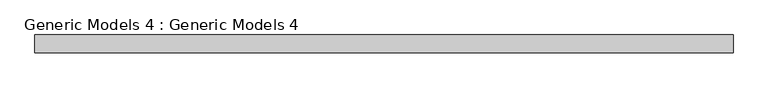
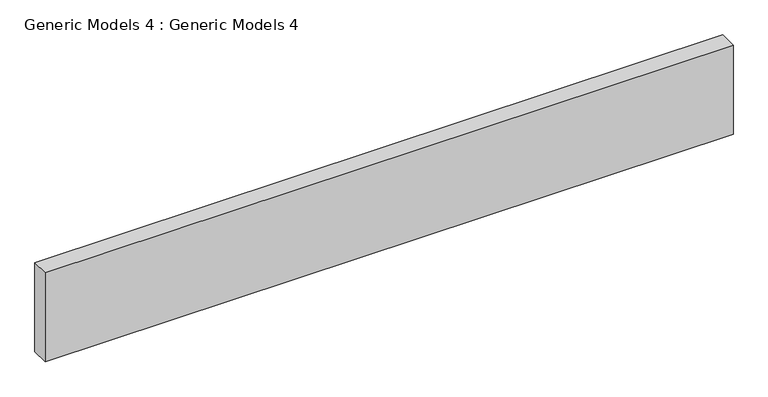
"""IFC4 building model written with IfcOpenShell, lengths in millimetres: proxy geometry, Generic Models 4 : Generic Models 4."""

from ifc_helpers import new_model, si_unit, frame, origin, place, context, project, spatial, polyline, outline, extrude, source, transform, mapped, element, save


def generic_models_4_generic_models_4_25668e5e(model_context):
    return source(origin(), model_context, "Body", "SweptSolid", [
        extrude(outline(polyline([(-10949.0161422, 5487.8132242), (-10949.0161422, 5259.2132242), (-19864.4161422, 5259.2132242), (-19864.4161422, 5487.8132242), (-10949.0161422, 5487.8132242)])), frame((0.0, 0.0, 6400.8), z_axis=(0.0, 0.0, 1.0), x_axis=(1.0, 0.0, 0.0)), (0.0, 0.0, 1.0), 1219.2),
    ])


if __name__ == "__main__":
    model = new_model("IFC4")
    model_context = context("Model", 3, world=origin())
    ifc_project = project(units=[si_unit("LENGTHUNIT", "METRE", prefix="MILLI")], contexts=[model_context])
    site = spatial("IfcSite", under=ifc_project)
    building = spatial("IfcBuilding", under=site)
    placement = place(None, origin())
    generic_models_4_generic_models_4_shape = generic_models_4_generic_models_4_25668e5e(model_context)
    element("IfcBuildingElementProxy", 1, Name="Generic Models 4 : Generic Models 4", ObjectType="Generic Models 4 : Generic Models 4", at=placement, inside=building, context=model_context, shape_type="MappedRepresentation", body=[
        mapped(generic_models_4_generic_models_4_shape, transform((0.0, 0.0, 0.0), x_axis=(1.0, 0.0, 0.0), y_axis=(0.0, 1.0, 0.0), z_axis=(0.0, 0.0, 1.0))),
    ])
    save(model, "model.ifc")
